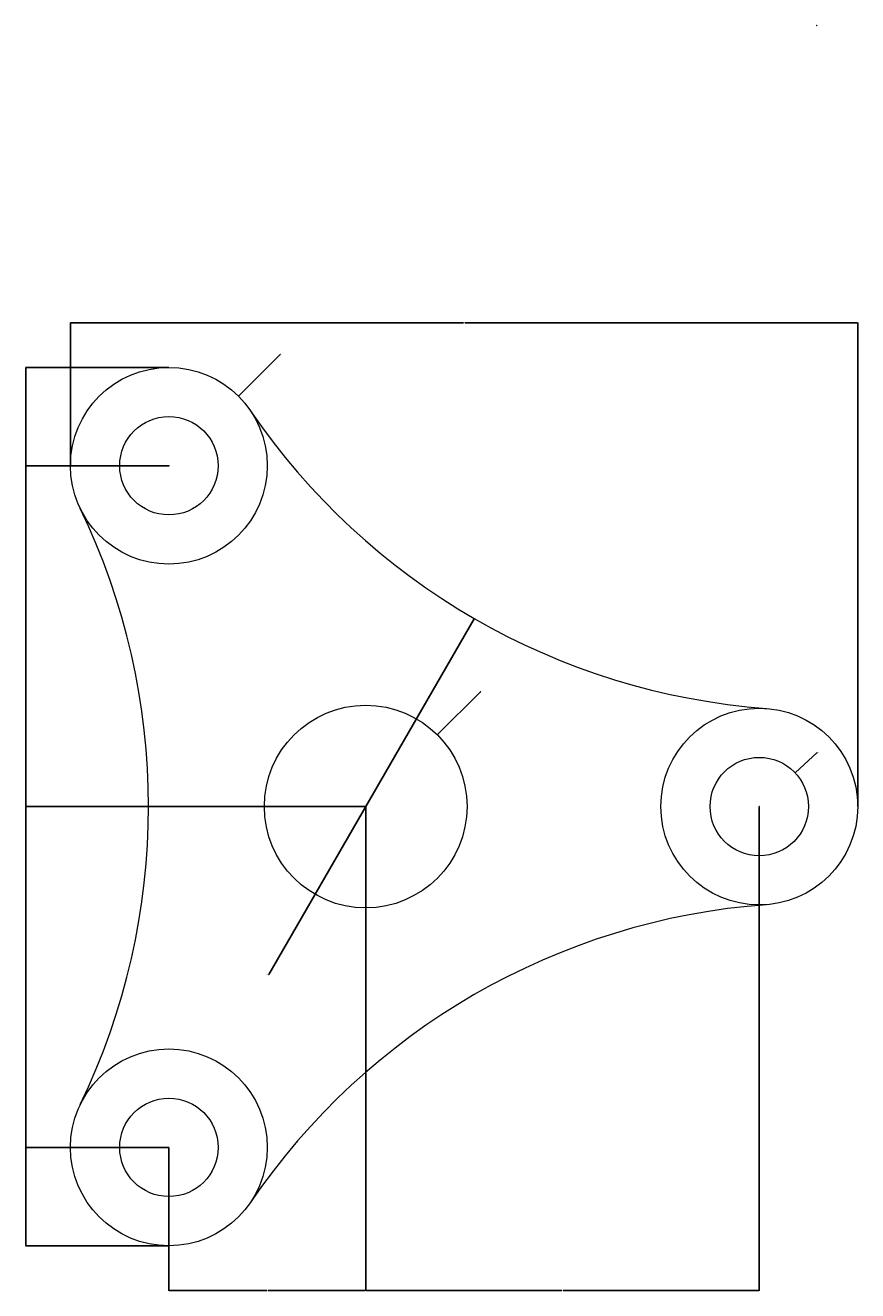
# Model space of a CAD drawing. Units: millimetres. Extents: x -15 to 2550, y 1225 to 3403.
# Tile 2 of 2: x 2127 to 2550, y 1225 to 1868. Entities that reach past the tile are written whole.
import ezdxf

# ---------------------------------------------------------------- set-up
doc = ezdxf.new("R2010")
doc.units = ezdxf.units.MM
doc.layers.add('M-CONS', color=7, linetype='Continuous', lineweight=18)
doc.layers.add('M-DIMS', color=2, linetype='Continuous', lineweight=18)
doc.styles.get("Standard").update_dxf_attribs({"font": 'arial.ttf'})
doc.dimstyles.get("Standard").update_dxf_attribs({"dimtxt": 0.18, "dimasz": 0.18, "dimexe": 0.18, "dimexo": 0.0625, "dimgap": 0.09, "dimtad": 0, "dimtih": 1, "dimtoh": 1, "dimdec": 4, "dimzin": 0, "dimdsep": 46, "dimtxsty": 'Standard', "dimcen": 0.09, "dimadec": 0, "dimazin": 0, "dimtfac": 1, "dimtdec": 4, "dimtofl": 0, "dimtmove": 0, "dimatfit": 3, "dimfxl": 1, "dimtolj": 1, "dimtzin": 0, "dimarcsym": 0})

# ---------------------------------------------------------------- blocks, each defined once
blk = doc.blocks.new('BOSS-PROFILE-100X50')
for radius in [50, 25]:
    blk.add_circle((0, 0), radius)
blk = doc.blocks.new('*D4')
at = {"layer": 'Defpoints', "color": 0, "transparency": 16777216}
for p in [(2300.25, 1471.27), (2200.25, 1298.06), (2300.25, 1225.41)]:
    blk.add_point(p, dxfattribs=at)
at = {"layer": 'M-DIMS', "color": 0, "lineweight": -2, "transparency": 16777216}
for p, q in [((2300.25, 1471.21), (2300.25, 1225.23)), ((2200.25, 1298), (2200.25, 1225.23)), ((2200.43, 1225.41), (2249.97, 1225.41)), ((2300.07, 1225.41), (2250.53, 1225.41))]:
    blk.add_line(p, q, dxfattribs=at)
at = {"layer": 'M-DIMS', "color": 0, "transparency": 16777216}
for points in [[(2200.43, 1225.44), (2200.43, 1225.38), (2200.25, 1225.41)], [(2300.07, 1225.44), (2300.07, 1225.38), (2300.25, 1225.41)]]:
    blk.add_solid(points, dxfattribs=at)
at = {"layer": 'M-DIMS', "color": 0, "transparency": 16777216, "insert": (2250.25, 1225.41), "char_height": 0.18, "attachment_point": 5}
blk.add_mtext('\\A1;100', dxfattribs=at)
blk = doc.blocks.new('*D5')
at = {"layer": 'Defpoints', "color": 0, "transparency": 16777216}
for p in [(2300.25, 1471.27), (2500.25, 1471.27), (2500.25, 1225.41)]:
    blk.add_point(p, dxfattribs=at)
at = {"layer": 'M-DIMS', "color": 0, "lineweight": -2, "transparency": 16777216}
for p, q in [((2300.25, 1471.21), (2300.25, 1225.23)), ((2500.25, 1471.21), (2500.25, 1225.23)), ((2300.43, 1225.41), (2399.96, 1225.41)), ((2500.07, 1225.41), (2400.54, 1225.41))]:
    blk.add_line(p, q, dxfattribs=at)
at = {"layer": 'M-DIMS', "color": 0, "transparency": 16777216}
for points in [[(2300.43, 1225.44), (2300.43, 1225.38), (2300.25, 1225.41)], [(2500.07, 1225.44), (2500.07, 1225.38), (2500.25, 1225.41)]]:
    blk.add_solid(points, dxfattribs=at)
at = {"layer": 'M-DIMS', "color": 0, "transparency": 16777216, "insert": (2400.25, 1225.41), "char_height": 0.18, "attachment_point": 5}
blk.add_mtext('\\A1;200', dxfattribs=at)
blk = doc.blocks.new('*D6')
at = {"layer": 'Defpoints', "color": 0, "transparency": 16777216}
for p in [(2127.6, 1471.27), (2300.25, 1471.27), (2200.25, 1298.06)]:
    blk.add_point(p, dxfattribs=at)
at = {"layer": 'M-DIMS', "color": 0, "lineweight": -2, "transparency": 16777216}
for p, q in [((2300.19, 1471.27), (2127.42, 1471.27)), ((2127.6, 1471.09), (2127.6, 1384.85)), ((2127.6, 1298.24), (2127.6, 1384.48)), ((2200.19, 1298.06), (2127.42, 1298.06))]:
    blk.add_line(p, q, dxfattribs=at)
at = {"layer": 'M-DIMS', "color": 0, "transparency": 16777216}
for points in [[(2127.57, 1471.09), (2127.63, 1471.09), (2127.6, 1471.27)], [(2127.57, 1298.24), (2127.63, 1298.24), (2127.6, 1298.06)]]:
    blk.add_solid(points, dxfattribs=at)
at = {"layer": 'M-DIMS', "color": 0, "transparency": 16777216, "insert": (2127.6, 1384.67), "char_height": 0.18, "attachment_point": 5}
blk.add_mtext('\\A1;173.2', dxfattribs=at)
blk = doc.blocks.new('*D7')
at = {"layer": 'Defpoints', "color": 0, "transparency": 16777216}
for p in [(2127.6, 1644.47), (2200.25, 1644.47), (2300.25, 1471.27)]:
    blk.add_point(p, dxfattribs=at)
at = {"layer": 'M-DIMS', "color": 0, "lineweight": -2, "transparency": 16777216}
for p, q in [((2200.19, 1644.47), (2127.42, 1644.47)), ((2127.6, 1644.29), (2127.6, 1558.05)), ((2127.6, 1471.45), (2127.6, 1557.69)), ((2300.19, 1471.27), (2127.42, 1471.27))]:
    blk.add_line(p, q, dxfattribs=at)
at = {"layer": 'M-DIMS', "color": 0, "transparency": 16777216}
for points in [[(2127.57, 1644.29), (2127.63, 1644.29), (2127.6, 1644.47)], [(2127.57, 1471.45), (2127.63, 1471.45), (2127.6, 1471.27)]]:
    blk.add_solid(points, dxfattribs=at)
at = {"layer": 'M-DIMS', "color": 0, "transparency": 16777216, "insert": (2127.6, 1557.87), "char_height": 0.18, "attachment_point": 5}
blk.add_mtext('\\A1;173.2', dxfattribs=at)
blk = doc.blocks.new('*D8')
at = {"layer": 'Defpoints', "color": 0, "transparency": 16777216}
for p in [(2550.25, 1717.12), (2150.25, 1644.47), (2550.25, 1471.27)]:
    blk.add_point(p, dxfattribs=at)
at = {"layer": 'M-DIMS', "color": 0, "lineweight": -2, "transparency": 16777216}
for p, q in [((2150.25, 1644.54), (2150.25, 1717.3)), ((2150.43, 1717.12), (2349.96, 1717.12)), ((2550.07, 1717.12), (2350.55, 1717.12)), ((2550.25, 1471.33), (2550.25, 1717.3))]:
    blk.add_line(p, q, dxfattribs=at)
at = {"layer": 'M-DIMS', "color": 0, "transparency": 16777216}
for points in [[(2150.43, 1717.15), (2150.43, 1717.09), (2150.25, 1717.12)], [(2550.07, 1717.15), (2550.07, 1717.09), (2550.25, 1717.12)]]:
    blk.add_solid(points, dxfattribs=at)
at = {"layer": 'M-DIMS', "color": 0, "transparency": 16777216, "insert": (2350.25, 1717.12), "char_height": 0.18, "attachment_point": 5}
blk.add_mtext('\\A1;400', dxfattribs=at)
blk = doc.blocks.new('*D9')
at = {"layer": 'Defpoints', "color": 0, "transparency": 16777216}
for p in [(2127.6, 1694.47), (2200.25, 1694.47), (2200.25, 1248.06)]:
    blk.add_point(p, dxfattribs=at)
at = {"layer": 'M-DIMS', "color": 0, "lineweight": -2, "transparency": 16777216}
for p, q in [((2200.19, 1694.47), (2127.42, 1694.47)), ((2127.6, 1694.29), (2127.6, 1471.45)), ((2127.6, 1248.24), (2127.6, 1471.09)), ((2200.19, 1248.06), (2127.42, 1248.06))]:
    blk.add_line(p, q, dxfattribs=at)
at = {"layer": 'M-DIMS', "color": 0, "transparency": 16777216}
for points in [[(2127.57, 1694.29), (2127.63, 1694.29), (2127.6, 1694.47)], [(2127.57, 1248.24), (2127.63, 1248.24), (2127.6, 1248.06)]]:
    blk.add_solid(points, dxfattribs=at)
at = {"layer": 'M-DIMS', "color": 0, "transparency": 16777216, "insert": (2127.6, 1471.27), "char_height": 0.18, "attachment_point": 5}
blk.add_mtext('\\A1;446.4', dxfattribs=at)
blk = doc.blocks.new('*D14')
at = {"layer": 'Defpoints', "color": 0, "transparency": 16777216}
for p in [(2529.42, 1868.2), (2355.42, 1566.82)]:
    blk.add_point(p, dxfattribs=at)
at = {"layer": 'M-DIMS', "color": 0, "lineweight": -2, "transparency": 16777216}
for p, q in [((2529.33, 1868.2), (2529.51, 1868.2)), ((2529.42, 1868.11), (2529.42, 1868.29)), ((2251.02, 1385.99), (2355.33, 1566.67)), ((2250.84, 1385.99), (2251.02, 1385.99))]:
    blk.add_line(p, q, dxfattribs=at)
at = {"layer": 'M-DIMS', "color": 0, "transparency": 16777216}
blk.add_solid([(2355.31, 1566.68), (2355.36, 1566.65), (2355.42, 1566.82)], dxfattribs=at)
at = {"layer": 'M-DIMS', "color": 0, "transparency": 16777216, "insert": (2250.27, 1385.99), "char_height": 0.18, "attachment_point": 5}
blk.add_mtext('\\A1;3X R348', dxfattribs=at)
blk = doc.blocks.new('*D15')
at = {"layer": 'Defpoints', "color": 0, "transparency": 16777216}
for p in [(2336.67, 1507.68), (2263.83, 1434.85)]:
    blk.add_point(p, dxfattribs=at)
at = {"layer": 'M-DIMS', "color": 0, "lineweight": -2, "transparency": 16777216}
for p, q in [((2358.52, 1529.53), (2336.8, 1507.81)), ((2358.7, 1529.53), (2358.52, 1529.53)), ((2300.16, 1471.27), (2300.34, 1471.27)), ((2300.25, 1471.18), (2300.25, 1471.36))]:
    blk.add_line(p, q, dxfattribs=at)
at = {"layer": 'M-DIMS', "color": 0, "transparency": 16777216}
blk.add_solid([(2336.78, 1507.83), (2336.82, 1507.79), (2336.67, 1507.68)], dxfattribs=at)
at = {"layer": 'M-DIMS', "color": 0, "transparency": 16777216, "insert": (2359.09, 1529.53), "char_height": 0.18, "attachment_point": 5}
blk.add_mtext('\\A1;∅103', dxfattribs=at)
blk = doc.blocks.new('*D16')
at = {"layer": 'Defpoints', "color": 0, "transparency": 16777216}
for p in [(2235.61, 1679.83), (2164.9, 1609.12)]:
    blk.add_point(p, dxfattribs=at)
at = {"layer": 'M-DIMS', "color": 0, "lineweight": -2, "transparency": 16777216}
for p, q in [((2256.82, 1701.04), (2235.74, 1679.96)), ((2257, 1701.04), (2256.82, 1701.04)), ((2200.16, 1644.47), (2200.34, 1644.47)), ((2200.25, 1644.38), (2200.25, 1644.56))]:
    blk.add_line(p, q, dxfattribs=at)
at = {"layer": 'M-DIMS', "color": 0, "transparency": 16777216}
blk.add_solid([(2235.71, 1679.98), (2235.76, 1679.93), (2235.61, 1679.83)], dxfattribs=at)
at = {"layer": 'M-DIMS', "color": 0, "transparency": 16777216, "insert": (2257.58, 1701.04), "char_height": 0.18, "attachment_point": 5}
blk.add_mtext('\\A1;3X ∅100', dxfattribs=at)
blk = doc.blocks.new('*D17')
at = {"layer": 'Defpoints', "color": 0, "transparency": 16777216}
for p in [(2518.48, 1488.38), (2482.03, 1454.16)]:
    blk.add_point(p, dxfattribs=at)
at = {"layer": 'M-DIMS', "color": 0, "lineweight": -2, "transparency": 16777216}
for p, q in [((2529.41, 1498.65), (2518.61, 1488.5)), ((2529.59, 1498.65), (2529.41, 1498.65)), ((2500.16, 1471.27), (2500.34, 1471.27)), ((2500.25, 1471.18), (2500.25, 1471.36))]:
    blk.add_line(p, q, dxfattribs=at)
at = {"layer": 'M-DIMS', "color": 0, "transparency": 16777216}
blk.add_solid([(2518.59, 1488.53), (2518.63, 1488.48), (2518.48, 1488.38)], dxfattribs=at)
at = {"layer": 'M-DIMS', "color": 0, "transparency": 16777216, "insert": (2530.1, 1498.65), "char_height": 0.18, "attachment_point": 5}
blk.add_mtext('\\A1;3X ∅50', dxfattribs=at)

msp = doc.modelspace()

# ---------------------------------------------------------------- linework, layer by layer
at = {"layer": 'M-CONS'}
msp.add_circle((2300.253, 1471.268), 51.5, dxfattribs=at)
for centre, start, end in [((2529.421, 1868.198), 214.202702, 265.797298), ((1841.918, 1471.268), 334.202702, 25.797298), ((2529.421, 1074.338), 94.202702, 145.797298)]:
    msp.add_arc(centre, 348, start, end, dxfattribs=at)

# ---------------------------------------------------------------- block references
for p in [(2200.253, 1644.473), (2500.253, 1471.268), (2200.253, 1298.063)]:
    msp.add_blockref('BOSS-PROFILE-100X50', p, dxfattribs=at)

# ---------------------------------------------------------------- dimensions: what is measured, and where the dimension line sits
at = {"layer": 'M-DIMS'}
dim = msp.add_radius_dim(center=(2529.421, 1868.198), mpoint=(2355.421, 1566.821), text='3X <>', dimstyle='Standard', override={"dimdec": 0, "dimlfac": 1, "dimrnd": 0, "dimzin": 0, "dimdsep": 46, "dimlunit": 2}, dxfattribs=at)
dim.commit()
dim.dimension.update_dxf_attribs({"geometry": '*D14', "text_midpoint": (2250.273, 1385.995), "dimtype": 164})
for base, p1, p2, picture, middle in [((2550.253, 1717.123), (2150.253, 1644.473), (2550.253, 1471.268), '*D8', (2350.253, 1717.123)), ((2300.253, 1225.413), (2200.253, 1298.063), (2300.253, 1471.268), '*D4', (2250.253, 1225.413)), ((2500.253, 1225.413), (2300.253, 1471.268), (2500.253, 1471.268), '*D5', (2400.253, 1225.413))]:
    dim = msp.add_linear_dim(base=base, p1=p1, p2=p2, dimstyle='Standard', override={"dimdec": 0, "dimlfac": 1, "dimrnd": 0, "dimzin": 0, "dimdsep": 46, "dimlunit": 2}, dxfattribs=at)
    dim.commit()
    dim.dimension.update_dxf_attribs({"geometry": picture, "text_midpoint": middle})
for p1, p2, picture, middle in [((2164.898, 1609.118), (2235.609, 1679.829), '*D16', (2257.577, 1701.042)), ((2482.028, 1454.156), (2518.479, 1488.38), '*D17', (2530.1, 1498.648))]:
    dim = msp.add_diameter_dim_2p(p1=p1, p2=p2, text='3X <>', dimstyle='Standard', override={"dimdec": 0, "dimlfac": 1, "dimrnd": 0, "dimzin": 0, "dimdsep": 46, "dimlunit": 2}, dxfattribs=at)
    dim.commit()
    dim.dimension.update_dxf_attribs({"geometry": picture, "text_midpoint": middle, "dimtype": 163})
for base, p1, p2, picture, middle in [((2127.603, 1694.473), (2200.253, 1248.063), (2200.253, 1694.473), '*D9', (2127.603, 1471.268)), ((2127.603, 1644.473), (2300.253, 1471.268), (2200.253, 1644.473), '*D7', (2127.603, 1557.871)), ((2127.603, 1471.268), (2200.253, 1298.063), (2300.253, 1471.268), '*D6', (2127.603, 1384.666))]:
    dim = msp.add_linear_dim(base=base, p1=p1, p2=p2, angle=90, dimstyle='Standard', override={"dimdec": 1, "dimlfac": 1, "dimrnd": 0, "dimzin": 0, "dimdsep": 46, "dimlunit": 2}, dxfattribs=at)
    dim.commit()
    dim.dimension.update_dxf_attribs({"geometry": picture, "text_midpoint": middle})
dim = msp.add_diameter_dim_2p(p1=(2263.835, 1434.855), p2=(2336.672, 1507.682), dimstyle='Standard', override={"dimdec": 0, "dimlfac": 1, "dimrnd": 0, "dimzin": 0, "dimdsep": 46, "dimlunit": 2}, dxfattribs=at)
dim.commit()
dim.dimension.update_dxf_attribs({"geometry": '*D15', "text_midpoint": (2359.09, 1529.53), "dimtype": 163})

doc.saveas('drawing.dxf')
